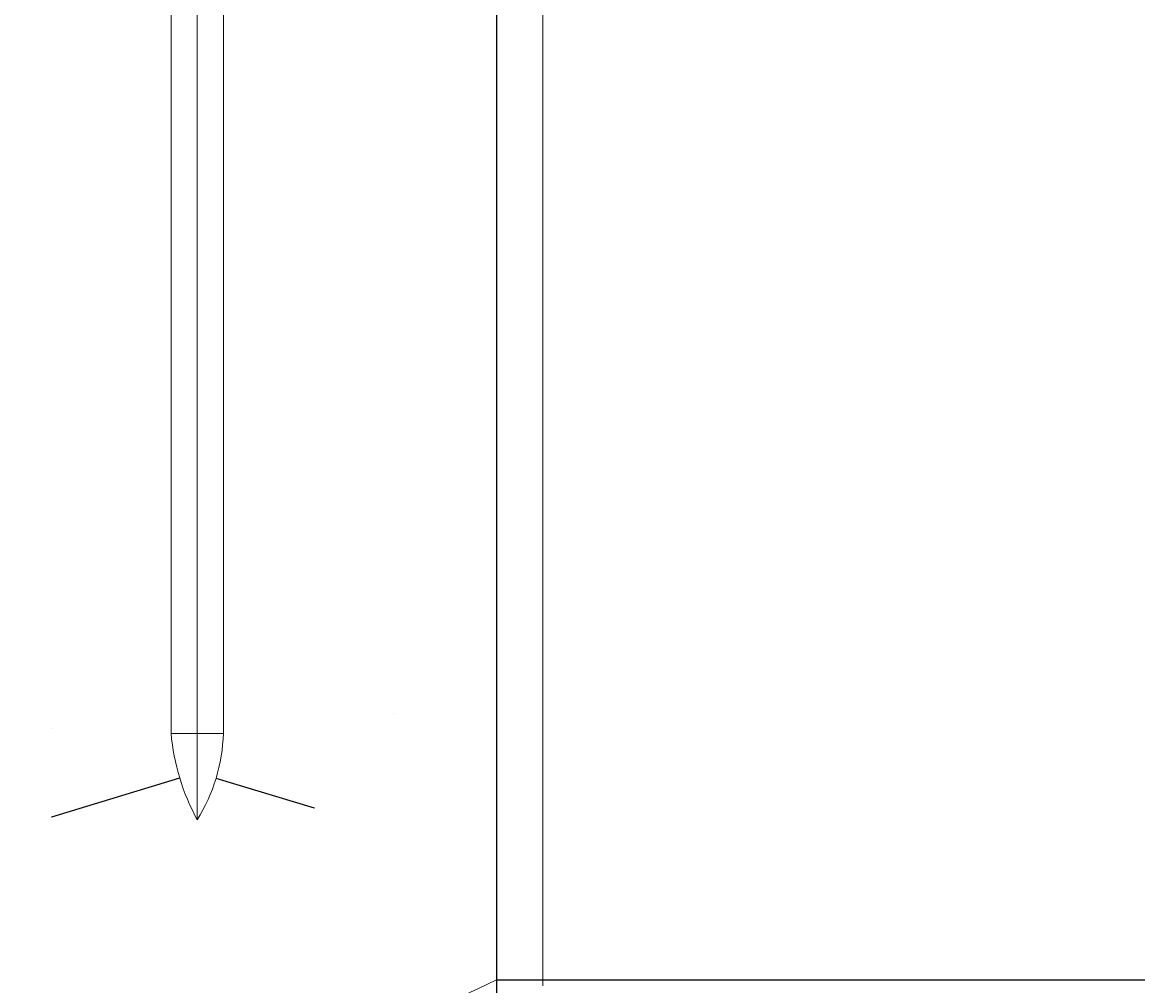
# Model space of a CAD drawing. Units: millimetres. Extents: x 353872 to 441597, y 126154 to 187356.
# Tile 9 of 28: x 394852 to 399262, y 141663 to 145472. Entities that reach past the tile are written whole.
import ezdxf

# ---------------------------------------------------------------- set-up
doc = ezdxf.new("R2010")
doc.units = ezdxf.units.MM
doc.layers.add('A-ANNO-DIMS', color=2, linetype='Continuous', lineweight=18)
doc.layers.add('P-INST-SIGN', color=4, linetype='Continuous', lineweight=18)
doc.styles.get("Standard").update_dxf_attribs({"font": 'arial.ttf'})
doc.dimstyles.get("Standard").update_dxf_attribs({"dimtxt": 0.18, "dimasz": 0.18, "dimexe": 0.18, "dimexo": 0.0625, "dimgap": 0.09, "dimtad": 0, "dimtih": 1, "dimtoh": 1, "dimdec": 4, "dimzin": 0, "dimdsep": 46, "dimtxsty": 'Standard', "dimcen": 0.09, "dimadec": 0, "dimazin": 0, "dimtfac": 1, "dimtdec": 4, "dimtofl": 0, "dimtmove": 0, "dimatfit": 3, "dimfxl": 1, "dimtolj": 1, "dimtzin": 0, "dimarcsym": 0})

# ---------------------------------------------------------------- blocks, each defined once
blk = doc.blocks.new('*D29')
at = {"layer": 'A-ANNO-DIMS', "color": 0, "lineweight": -2, "transparency": 16777216}
for p, q in [((391689.9, 148464.5), (391689.9, 133812.7)), ((396727.5, 148464.5), (396727.5, 133812.7)), ((391690.1, 133812.8), (394208.4, 133812.8)), ((396727.3, 133812.8), (394209.1, 133812.8))]:
    blk.add_line(p, q, dxfattribs=at)
at = {"layer": 'A-ANNO-DIMS', "color": 0, "transparency": 16777216}
for points in [[(391690.1, 133812.9), (391690.1, 133812.8), (391689.9, 133812.8)], [(396727.3, 133812.9), (396727.3, 133812.8), (396727.5, 133812.8)]]:
    blk.add_solid(points, dxfattribs=at)
at = {"layer": 'Defpoints', "color": 0, "transparency": 16777216}
for p in [(391689.9, 148464.5), (396727.5, 148464.5), (396727.5, 133812.8)]:
    blk.add_point(p, dxfattribs=at)
at = {"layer": 'A-ANNO-DIMS', "color": 0, "transparency": 16777216, "insert": (394208.7, 133812.8), "char_height": 0.18, "attachment_point": 5}
blk.add_mtext('\\A1;5038', dxfattribs=at)
blk = doc.blocks.new('*D30')
at = {"layer": 'A-ANNO-DIMS', "color": 0, "lineweight": -2, "transparency": 16777216}
for p, q in [((396727.6, 148464.5), (440591.2, 148464.5)), ((440591, 148464.3), (440591, 145075.4)), ((440591, 141686), (440591, 145075)), ((396727.6, 141685.8), (440591.2, 141685.8))]:
    blk.add_line(p, q, dxfattribs=at)
at = {"layer": 'A-ANNO-DIMS', "color": 0, "transparency": 16777216}
for points in [[(440591, 148464.3), (440591, 148464.3), (440591, 148464.5)], [(440591, 141686), (440591, 141686), (440591, 141685.8)]]:
    blk.add_solid(points, dxfattribs=at)
at = {"layer": 'Defpoints', "color": 0, "transparency": 16777216}
for p in [(396727.5, 148464.5), (396727.5, 141685.8), (440591, 141685.8)]:
    blk.add_point(p, dxfattribs=at)
at = {"layer": 'A-ANNO-DIMS', "color": 0, "transparency": 16777216, "insert": (440591, 145075.2), "char_height": 0.18, "attachment_point": 5}
blk.add_mtext('\\A1;6779', dxfattribs=at)
blk = doc.blocks.new('*D38')
at = {"layer": 'A-ANNO-DIMS', "color": 0, "lineweight": -2, "transparency": 16777216}
for p, q in [((396318.3, 142739.8), (396318.3, 142740)), ((396318.3, 142739.9), (396318.4, 142739.9)), ((394968.6, 142330.8), (395474.6, 142484.2)), ((394968.4, 142330.8), (394968.6, 142330.8))]:
    blk.add_line(p, q, dxfattribs=at)
at = {"layer": 'A-ANNO-DIMS', "color": 0, "transparency": 16777216}
blk.add_solid([(395474.5, 142484.2), (395474.6, 142484.1), (395474.7, 142484.2)], dxfattribs=at)
at = {"layer": 'Defpoints', "color": 0, "transparency": 16777216}
for p in [(396318.3, 142739.9), (395474.7, 142484.2)]:
    blk.add_point(p, dxfattribs=at)
at = {"layer": 'A-ANNO-DIMS', "color": 0, "transparency": 16777216, "insert": (394967.9, 142330.8), "char_height": 0.18, "attachment_point": 5}
blk.add_mtext('\\A1;R881.5', dxfattribs=at)
blk = doc.blocks.new('*D39')
at = {"layer": 'A-ANNO-DIMS', "color": 0, "lineweight": -2, "transparency": 16777216}
for p, q in [((394968.8, 142679.4), (394969, 142679.4)), ((394968.9, 142679.3), (394968.9, 142679.5)), ((396008, 142364.5), (395618.5, 142482.5)), ((396008.2, 142364.5), (396008, 142364.5))]:
    blk.add_line(p, q, dxfattribs=at)
at = {"layer": 'A-ANNO-DIMS', "color": 0, "transparency": 16777216}
blk.add_solid([(395618.5, 142482.6), (395618.5, 142482.5), (395618.3, 142482.6)], dxfattribs=at)
at = {"layer": 'Defpoints', "color": 0, "transparency": 16777216}
for p in [(394968.9, 142679.4), (395618.3, 142482.6)]:
    blk.add_point(p, dxfattribs=at)
at = {"layer": 'A-ANNO-DIMS', "color": 0, "transparency": 16777216, "insert": (396008.7, 142364.5), "char_height": 0.18, "attachment_point": 5}
blk.add_mtext('\\A1;R678.6', dxfattribs=at)

msp = doc.modelspace()

# ---------------------------------------------------------------- linework, layer by layer
at = {"layer": 'P-INST-SIGN'}
for p, q in [((395543.84, 149129.17), (395543.84, 142318.92)), ((395440.46, 149056.78), (395440.46, 142660.1)), ((395647.23, 149056.78), (395647.23, 142660.1)), ((395440.46, 142660.1), (395647.23, 142660.1))]:
    msp.add_line(p, q, dxfattribs=at)
for points in [[(396727.53, 148464.52), (396727.53, 148464.52), (396727.53, 141685.82)], [(396910.35, 147126.17), (396910.35, 141662.82)]]:
    msp.add_lwpolyline(points, dxfattribs=at)
for centre, radius, start, end in [((396318.34, 142739.87), 881.51, 185.19226, 208.52461), ((394968.87, 142679.41), 678.63, 327.91374, 358.36939), ((394208.72, 146860.25), 5754.92, 244.04409, 295.95591)]:
    msp.add_arc(centre, radius, start, end, dxfattribs=at)

# ---------------------------------------------------------------- dimensions: what is measured, and where the dimension line sits
at = {"layer": 'A-ANNO-DIMS'}
dim = msp.add_linear_dim(base=(396727.53, 133812.84), p1=(391689.9, 148464.52), p2=(396727.53, 148464.52), dimstyle='Standard', override={"dimdec": 0, "dimlfac": 1, "dimrnd": 0, "dimzin": 0, "dimdsep": 46, "dimlunit": 2}, dxfattribs=at)
dim.commit()
dim.dimension.update_dxf_attribs({"geometry": '*D29', "text_midpoint": (394208.72, 133812.84)})
dim = msp.add_linear_dim(base=(440591, 141685.82), p1=(396727.53, 148464.52), p2=(396727.53, 141685.82), angle=90, dimstyle='Standard', override={"dimdec": 0, "dimlfac": 1, "dimrnd": 0, "dimzin": 0, "dimdsep": 46, "dimlunit": 2}, dxfattribs=at)
dim.commit()
dim.dimension.update_dxf_attribs({"geometry": '*D30', "text_midpoint": (440591, 145075.17)})
for center, mpoint, picture, middle in [((396318.34, 142739.87), (395474.73, 142484.21), '*D38', (394967.9, 142330.81)), ((394968.87, 142679.41), (395618.34, 142482.59), '*D39', (396008.68, 142364.5))]:
    dim = msp.add_radius_dim(center=center, mpoint=mpoint, dimstyle='Standard', override={"dimdec": 1, "dimlfac": 1, "dimrnd": 0, "dimzin": 0, "dimdsep": 46, "dimlunit": 2}, dxfattribs=at)
    dim.commit()
    dim.dimension.update_dxf_attribs({"geometry": picture, "text_midpoint": middle, "dimtype": 164})

doc.saveas('drawing.dxf')
